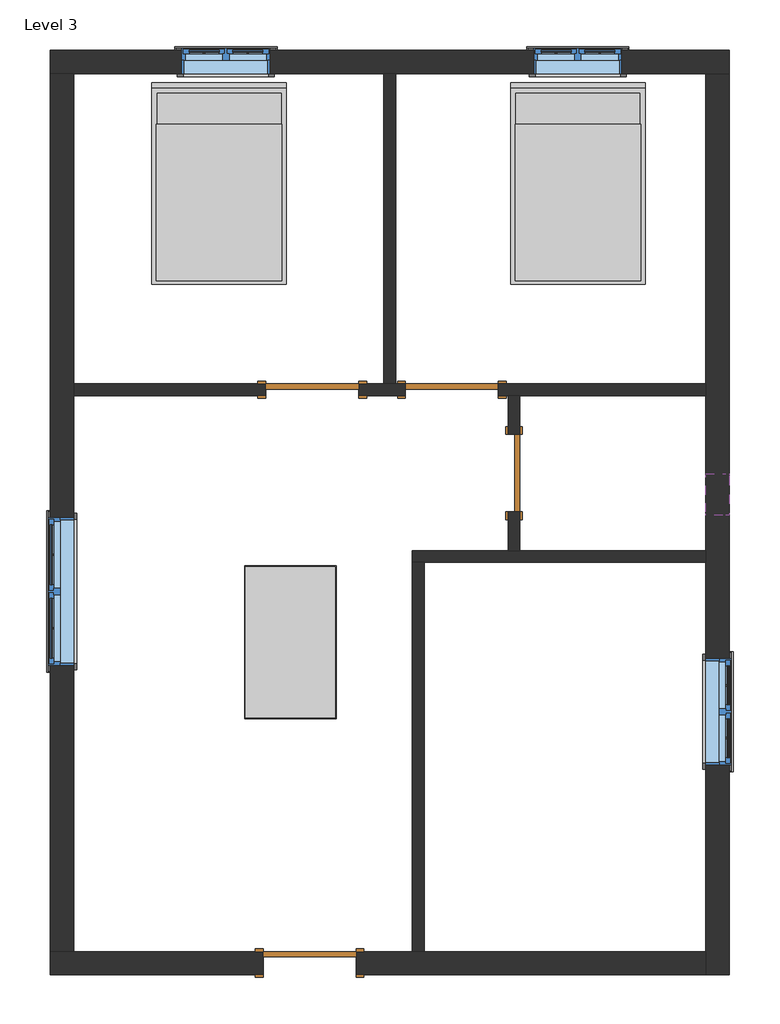
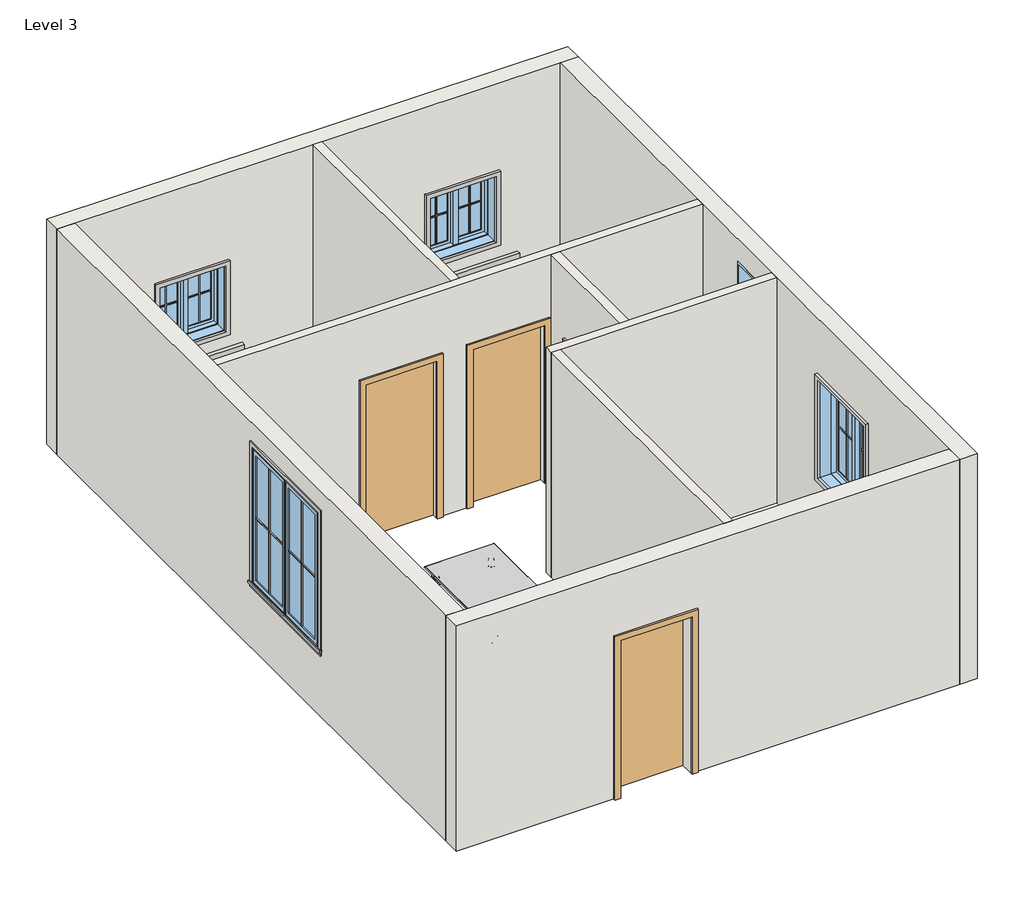
# One storey, incomplete: 16 proxies, 9 walls, 5 windows, 4 doors, 3 furniture elements.
"""IFC4 building model written with IfcOpenShell, lengths in millimetres."""

from ifc_helpers import new_model, si_unit, frame, origin, place, context, project, spatial, polyline, outline, extrude, faceted_brep, transform, mapped, element, save
from components import muntin_pattern_2x2_muntin_pattern_2x2_b3fe6957, muntin_pattern_2x2_muntin_pattern_2x2_3e0ecaf2, muntin_pattern_2x2_muntin_pattern_2x2_bff912c5, muntin_pattern_2x2_muntin_pattern_2x2_c2194282, muntin_pattern_2x2_muntin_pattern_2x2_88bf7f41, muntin_pattern_2x2_muntin_pattern_2x2_3dfd0a47, trim_window_exterior_flat_with_sill_41619996, trim_window_exterior_flat_with_sill_e04b3088, trim_window_exterior_flat_with_sill_4930676f, trim_window_interior_flat_picture_frame_51c85655, trim_window_interior_flat_picture_frame_2a7685fe, trim_window_interior_flat_picture_frame_dd064338, door_f2b275c1, door_e5f9f3c4, door_305aa2a5, door_0ca8825f, bed_17739_bed_17739_15c61121, dining_table_14755_dining_table_14755_d89cb775, window_aa618e30, window_339605e1, window_c95ebb39, window_9ac97e1a

model = new_model("IFC4")

# Units and contexts
model_context = context("Model", 3, world=origin())
ifc_project = project(units=[si_unit("LENGTHUNIT", "METRE", prefix="MILLI")], contexts=[model_context])

# Site, building, storey
site = spatial("IfcSite", under=ifc_project)
building = spatial("IfcBuilding", under=site)
storey = spatial("IfcBuildingStorey", under=building, Name="Level 3", Elevation=3200.4)

# Proxies
placement = place(None, origin())
muntin_pattern_2x2_muntin_pattern_2x2_shape = muntin_pattern_2x2_muntin_pattern_2x2_b3fe6957(model_context)
element("IfcBuildingElementProxy", 1, Name="Muntin Pattern_2x2 : Muntin Pattern_2x2", ObjectType="Muntin Pattern_2x2 : Muntin Pattern_2x2", at=placement, inside=storey, context=model_context, shape_type="MappedRepresentation", body=[
    mapped(muntin_pattern_2x2_muntin_pattern_2x2_shape, transform((-3079.2790084, 5068.9185985, 4184.65), x_axis=(1.0, 0.0, 0.0), y_axis=(0.0, 1.0, 0.0), z_axis=(0.0, 0.0, 1.0))),
])
element("IfcBuildingElementProxy", 2, Name="Muntin Pattern_2x2 : Muntin Pattern_2x2", ObjectType="Muntin Pattern_2x2 : Muntin Pattern_2x2", at=placement, inside=storey, context=model_context, shape_type="MappedRepresentation", body=[
    mapped(muntin_pattern_2x2_muntin_pattern_2x2_shape, transform((378.2959916, 5068.9185985, 4184.65), x_axis=(1.0, 0.0, 0.0), y_axis=(0.0, 1.0, 0.0), z_axis=(0.0, 0.0, 1.0))),
])
muntin_pattern_2x2_muntin_pattern_2x2_2_shape = muntin_pattern_2x2_muntin_pattern_2x2_3e0ecaf2(model_context)
element("IfcBuildingElementProxy", 3, Name="Muntin Pattern_2x2 : Muntin Pattern_2x2", ObjectType="Muntin Pattern_2x2 : Muntin Pattern_2x2", at=placement, inside=storey, context=model_context, shape_type="MappedRepresentation", body=[
    mapped(muntin_pattern_2x2_muntin_pattern_2x2_2_shape, transform((-2650.6540084, 5068.9185985, 4184.65), x_axis=(-1.0, 0.0, 0.0), y_axis=(0.0, -1.0, 0.0), z_axis=(0.0, 0.0, 1.0))),
])
element("IfcBuildingElementProxy", 4, Name="Muntin Pattern_2x2 : Muntin Pattern_2x2", ObjectType="Muntin Pattern_2x2 : Muntin Pattern_2x2", at=placement, inside=storey, context=model_context, shape_type="MappedRepresentation", body=[
    mapped(muntin_pattern_2x2_muntin_pattern_2x2_2_shape, transform((806.9209916, 5068.9185985, 4184.65), x_axis=(-1.0, 0.0, 0.0), y_axis=(0.0, -1.0, 0.0), z_axis=(0.0, 0.0, 1.0))),
])
muntin_pattern_2x2_muntin_pattern_2x2_3_shape = muntin_pattern_2x2_muntin_pattern_2x2_bff912c5(model_context)
element("IfcBuildingElementProxy", 5, Name="Muntin Pattern_2x2 : Muntin Pattern_2x2", ObjectType="Muntin Pattern_2x2 : Muntin Pattern_2x2", at=placement, inside=storey, context=model_context, shape_type="MappedRepresentation", body=[
    mapped(muntin_pattern_2x2_muntin_pattern_2x2_3_shape, transform((-4579.4665084, -596.8689015, 4184.65), x_axis=(0.0, 1.0, 0.0), y_axis=(-1.0, 0.0, 0.0), z_axis=(0.0, 0.0, 1.0))),
])
muntin_pattern_2x2_muntin_pattern_2x2_4_shape = muntin_pattern_2x2_muntin_pattern_2x2_c2194282(model_context)
element("IfcBuildingElementProxy", 6, Name="Muntin Pattern_2x2 : Muntin Pattern_2x2", ObjectType="Muntin Pattern_2x2 : Muntin Pattern_2x2", at=placement, inside=storey, context=model_context, shape_type="MappedRepresentation", body=[
    mapped(muntin_pattern_2x2_muntin_pattern_2x2_4_shape, transform((-4579.4665084, 123.8560985, 4184.65), x_axis=(0.0, -1.0, 0.0), y_axis=(1.0, 0.0, 0.0), z_axis=(0.0, 0.0, 1.0))),
])
muntin_pattern_2x2_muntin_pattern_2x2_5_shape = muntin_pattern_2x2_muntin_pattern_2x2_88bf7f41(model_context)
element("IfcBuildingElementProxy", 7, Name="Muntin Pattern_2x2 : Muntin Pattern_2x2", ObjectType="Muntin Pattern_2x2 : Muntin Pattern_2x2", at=placement, inside=storey, context=model_context, shape_type="MappedRepresentation", body=[
    mapped(muntin_pattern_2x2_muntin_pattern_2x2_5_shape, transform((2068.9834916, -1158.8439015, 4184.65), x_axis=(0.0, -1.0, 0.0), y_axis=(1.0, 0.0, 0.0), z_axis=(0.0, 0.0, 1.0))),
])
muntin_pattern_2x2_muntin_pattern_2x2_6_shape = muntin_pattern_2x2_muntin_pattern_2x2_3dfd0a47(model_context)
element("IfcBuildingElementProxy", 8, Name="Muntin Pattern_2x2 : Muntin Pattern_2x2", ObjectType="Muntin Pattern_2x2 : Muntin Pattern_2x2", at=placement, inside=storey, context=model_context, shape_type="MappedRepresentation", body=[
    mapped(muntin_pattern_2x2_muntin_pattern_2x2_6_shape, transform((2068.9834916, -1676.3689015, 4184.65), x_axis=(0.0, 1.0, 0.0), y_axis=(-1.0, 0.0, 0.0), z_axis=(0.0, 0.0, 1.0))),
])
trim_window_exterior_flat_with_sill_shape = trim_window_exterior_flat_with_sill_41619996(model_context)
element("IfcBuildingElementProxy", 9, Name="Trim-Window-Exterior-Flat : with Sill", ObjectType="Trim-Window-Exterior-Flat : with Sill", at=placement, inside=storey, context=model_context, shape_type="MappedRepresentation", body=[
    mapped(trim_window_exterior_flat_with_sill_shape, transform((-2864.9665084, 5078.4435985, 5029.2), x_axis=(-1.0, 0.0, 0.0), y_axis=(0.0, 0.0, 1.0), z_axis=(0.0, 1.0, 0.0))),
])
element("IfcBuildingElementProxy", 10, Name="Trim-Window-Exterior-Flat : with Sill", ObjectType="Trim-Window-Exterior-Flat : with Sill", at=placement, inside=storey, context=model_context, shape_type="MappedRepresentation", body=[
    mapped(trim_window_exterior_flat_with_sill_shape, transform((592.6084916, 5078.4435985, 5029.2), x_axis=(-1.0, 0.0, 0.0), y_axis=(0.0, 0.0, 1.0), z_axis=(0.0, 1.0, 0.0))),
])
trim_window_exterior_flat_with_sill_2_shape = trim_window_exterior_flat_with_sill_e04b3088(model_context)
element("IfcBuildingElementProxy", 11, Name="Trim-Window-Exterior-Flat : with Sill", ObjectType="Trim-Window-Exterior-Flat : with Sill", at=placement, inside=storey, context=model_context, shape_type="MappedRepresentation", body=[
    mapped(trim_window_exterior_flat_with_sill_2_shape, transform((-4588.9915084, -236.5064015, 5943.6), x_axis=(0.0, -1.0, 0.0), y_axis=(0.0, 0.0, 1.0), z_axis=(-1.0, 0.0, 0.0))),
])
trim_window_exterior_flat_with_sill_3_shape = trim_window_exterior_flat_with_sill_4930676f(model_context)
element("IfcBuildingElementProxy", 12, Name="Trim-Window-Exterior-Flat : with Sill", ObjectType="Trim-Window-Exterior-Flat : with Sill", at=placement, inside=storey, context=model_context, shape_type="MappedRepresentation", body=[
    mapped(trim_window_exterior_flat_with_sill_3_shape, transform((2078.5084916, -1417.6064015, 5461.0), x_axis=(0.0, 1.0, 0.0), y_axis=(0.0, 0.0, 1.0), z_axis=(1.0, 0.0, 0.0))),
])
trim_window_interior_flat_picture_frame_shape = trim_window_interior_flat_picture_frame_51c85655(model_context)
element("IfcBuildingElementProxy", 13, Name="Trim-Window-Interior-Flat : Picture Frame", ObjectType="Trim-Window-Interior-Flat : Picture Frame", at=placement, inside=storey, context=model_context, shape_type="MappedRepresentation", body=[
    mapped(trim_window_interior_flat_picture_frame_shape, transform((-2864.9665084, 4849.8435985, 5029.2), x_axis=(1.0, 0.0, 0.0), y_axis=(0.0, 0.0, 1.0), z_axis=(0.0, -1.0, 0.0))),
])
element("IfcBuildingElementProxy", 14, Name="Trim-Window-Interior-Flat : Picture Frame", ObjectType="Trim-Window-Interior-Flat : Picture Frame", at=placement, inside=storey, context=model_context, shape_type="MappedRepresentation", body=[
    mapped(trim_window_interior_flat_picture_frame_shape, transform((592.6084916, 4849.8435985, 5029.2), x_axis=(1.0, 0.0, 0.0), y_axis=(0.0, 0.0, 1.0), z_axis=(0.0, -1.0, 0.0))),
])
trim_window_interior_flat_picture_frame_2_shape = trim_window_interior_flat_picture_frame_2a7685fe(model_context)
element("IfcBuildingElementProxy", 15, Name="Trim-Window-Interior-Flat : Picture Frame", ObjectType="Trim-Window-Interior-Flat : Picture Frame", at=placement, inside=storey, context=model_context, shape_type="MappedRepresentation", body=[
    mapped(trim_window_interior_flat_picture_frame_2_shape, transform((-4360.3915084, -236.5064015, 5943.6), x_axis=(0.0, 1.0, 0.0), y_axis=(0.0, 0.0, 1.0), z_axis=(1.0, 0.0, 0.0))),
])
trim_window_interior_flat_picture_frame_3_shape = trim_window_interior_flat_picture_frame_dd064338(model_context)
element("IfcBuildingElementProxy", 16, Name="Trim-Window-Interior-Flat : Picture Frame", ObjectType="Trim-Window-Interior-Flat : Picture Frame", at=placement, inside=storey, context=model_context, shape_type="MappedRepresentation", body=[
    mapped(trim_window_interior_flat_picture_frame_3_shape, transform((1849.9084916, -1417.6064015, 5461.0), x_axis=(0.0, -1.0, 0.0), y_axis=(0.0, 0.0, 1.0), z_axis=(-1.0, 0.0, 0.0))),
])

# Doors
door_shape = door_f2b275c1(model_context)
element("IfcDoor", 17, ObjectType="Single-Flush : 30\" x 80\"", at=placement, inside=storey, context=model_context, shape_type="MappedRepresentation", body=[
    mapped(door_shape, transform((-36.0415084, 925.5435985, 3200.4), x_axis=(0.0, 1.0, 0.0), y_axis=(-1.0, 0.0, 0.0), z_axis=(0.0, 0.0, 1.0))),
])
door_2_shape = door_e5f9f3c4(model_context)
element("IfcDoor", 18, ObjectType="Single-Flush : 36\" x 84\"", at=placement, inside=storey, context=model_context, shape_type="MappedRepresentation", body=[
    mapped(door_2_shape, transform((-2017.2415084, 1744.6935985, 3200.4), x_axis=(1.0, 0.0, 0.0), y_axis=(0.0, 1.0, 0.0), z_axis=(0.0, 0.0, 1.0))),
])
door_3_shape = door_305aa2a5(model_context)
element("IfcDoor", 19, ObjectType="Single-Flush : 36\" x 84\"", at=placement, inside=storey, context=model_context, shape_type="MappedRepresentation", body=[
    mapped(door_3_shape, transform((-645.6415084, 1744.6935985, 3200.4), x_axis=(-1.0, 0.0, 0.0), y_axis=(0.0, -1.0, 0.0), z_axis=(0.0, 0.0, 1.0))),
])
door_4_shape = door_0ca8825f(model_context)
element("IfcDoor", 20, ObjectType="Single-Flush : 36\" x 84\"", at=placement, inside=storey, context=model_context, shape_type="MappedRepresentation", body=[
    mapped(door_4_shape, transform((-2042.6415084, -3887.7564015, 3200.4), x_axis=(1.0, 0.0, 0.0), y_axis=(0.0, 1.0, 0.0), z_axis=(0.0, 0.0, 1.0))),
])

# Furniture
bed_17739_bed_17739_shape = bed_17739_bed_17739_15c61121(model_context)
element("IfcFurniture", 21, ObjectType="Bed_17739 : Bed_17739", at=placement, inside=storey, context=model_context, shape_type="MappedRepresentation", body=[
    mapped(bed_17739_bed_17739_shape, transform((-2931.6415084, 3744.9435985, 3200.4), x_axis=(1.0, 0.0, 0.0), y_axis=(0.0, 1.0, 0.0), z_axis=(0.0, 0.0, 1.0))),
])
element("IfcFurniture", 22, ObjectType="Bed_17739 : Bed_17739", at=placement, inside=storey, context=model_context, shape_type="MappedRepresentation", body=[
    mapped(bed_17739_bed_17739_shape, transform((592.6084916, 3744.9435985, 3200.4), x_axis=(1.0, 0.0, 0.0), y_axis=(0.0, 1.0, 0.0), z_axis=(0.0, 0.0, 1.0))),
])
dining_table_14755_dining_table_14755_shape = dining_table_14755_dining_table_14755_d89cb775(model_context)
element("IfcFurniture", 23, ObjectType="Dining_table_14755 : Dining_table_14755", at=placement, inside=storey, context=model_context, shape_type="MappedRepresentation", body=[
    mapped(dining_table_14755_dining_table_14755_shape, transform((-1781.6222109, -1485.4350296, 3200.4), x_axis=(0.0, 1.0, 0.0), y_axis=(-1.0, 0.0, 0.0), z_axis=(0.0, 0.0, 1.0))),
])

# Walls
element("IfcWall", 24, ObjectType="WALL4.5\"", at=placement, inside=storey, context=model_context, shape_type="Brep", body=[
    faceted_brep([(-1560.0415084, 1687.5435985, 3200.4), (-1102.8415084, 1687.5435985, 3200.4), (-1102.8415084, 1687.5435985, 5334.0), (-188.4415084, 1687.5435985, 5334.0), (-188.4415084, 1687.5435985, 3200.4), (-93.1915084, 1687.5435985, 3200.4), (21.1084916, 1687.5435985, 3200.4), (1849.9084916, 1687.5435985, 3200.4), (1849.9084916, 1687.5435985, 6248.4), (21.1084916, 1687.5435985, 6248.4), (-93.1915084, 1687.5435985, 6248.4), (-4360.3915084, 1687.5435985, 6248.4), (-4360.3915084, 1687.5435985, 3200.4), (-2474.4415084, 1687.5435985, 3200.4), (-2474.4415084, 1687.5435985, 5334.0), (-1560.0415084, 1687.5435985, 5334.0), (-1102.8415084, 1801.8435985, 5334.0), (-1102.8415084, 1801.8435985, 3200.4), (-1198.0915084, 1801.8435985, 3200.4), (-1312.3915084, 1801.8435985, 3200.4), (-1560.0415084, 1801.8435985, 3200.4), (-1560.0415084, 1801.8435985, 5334.0), (-2474.4415084, 1801.8435985, 5334.0), (-2474.4415084, 1801.8435985, 3200.4), (-4360.3915084, 1801.8435985, 3200.4), (-4360.3915084, 1801.8435985, 6248.4), (-1312.3915084, 1801.8435985, 6248.4), (-1198.0915084, 1801.8435985, 6248.4), (1849.9084916, 1801.8435985, 6248.4), (1849.9084916, 1801.8435985, 3200.4), (-188.4415084, 1801.8435985, 3200.4), (-188.4415084, 1801.8435985, 5334.0)], [[[0, 1, 2, 3, 4, 5, 6, 7, 8, 9, 10, 11, 12, 13, 14, 15]], [[16, 17, 18, 19, 20, 21, 22, 23, 24, 25, 26, 27, 28, 29, 30, 31]], [[13, 12, 24, 23]], [[30, 29, 7, 6, 5, 4]], [[20, 19, 18, 17, 1, 0]], [[8, 7, 29, 28]], [[12, 11, 25, 24]], [[21, 20, 0, 15]], [[22, 21, 15, 14]], [[23, 22, 14, 13]], [[2, 1, 17, 16]], [[3, 2, 16, 31]], [[4, 3, 31, 30]], [[11, 10, 9, 8, 28, 27, 26, 25]]]),
])
element("IfcWall", 25, ObjectType="WALL4.5\"", at=placement, inside=storey, context=model_context, shape_type="SweptSolid", body=[
    extrude(outline(polyline([(-1312.3915084, 1801.8435985), (-1312.3915084, 4849.8435985), (-1198.0915084, 4849.8435985), (-1198.0915084, 1801.8435985), (-1312.3915084, 1801.8435985)])), frame((0.0, 0.0, 3200.4), z_axis=(0.0, 0.0, 1.0), x_axis=(1.0, 0.0, 0.0)), (0.0, 0.0, 1.0), 3048.0),
])
element("IfcWall", 26, ObjectType="WALL4.5\"", at=placement, inside=storey, context=model_context, shape_type="SweptSolid", body=[
    extrude(outline(polyline([(1687.5435985, 3200.4), (1306.5435985, 3200.4), (1306.5435985, 5232.4), (544.5435985, 5232.4), (544.5435985, 3200.4), (163.5435985, 3200.4), (163.5435985, 6248.4), (1687.5435985, 6248.4), (1687.5435985, 3200.4)])), frame((-93.1915084, 0.0, 0.0), z_axis=(1.0, 0.0, 0.0), x_axis=(0.0, 1.0, 0.0)), (0.0, 0.0, 1.0), 114.3),
])
element("IfcWall", 27, ObjectType="WALL4.5\"", at=placement, inside=storey, context=model_context, shape_type="Brep", body=[
    faceted_brep([(1849.9084916, 163.5435985, 3200.4), (21.1084916, 163.5435985, 3200.4), (-93.1915084, 163.5435985, 3200.4), (-1032.9915084, 163.5435985, 3200.4), (-1032.9915084, 163.5435985, 6248.4), (-93.1915084, 163.5435985, 6248.4), (21.1084916, 163.5435985, 6248.4), (1849.9084916, 163.5435985, 6248.4), (1849.9084916, 49.2435985, 3200.4), (1849.9084916, 49.2435985, 6248.4), (-918.6915084, 49.2435985, 6248.4), (-1032.9915084, 49.2435985, 6248.4), (-1032.9915084, 49.2435985, 3200.4), (-918.6915084, 49.2435985, 3200.4)], [[[0, 1, 2, 3, 4, 5, 6, 7]], [[8, 9, 10, 11, 12, 13]], [[3, 2, 1, 0, 8, 13, 12]], [[0, 7, 9, 8]], [[4, 3, 12, 11]], [[7, 6, 5, 4, 11, 10, 9]]]),
])
element("IfcWall", 28, ObjectType="WALL4.5\"", at=placement, inside=storey, context=model_context, shape_type="SweptSolid", body=[
    extrude(outline(polyline([(-1032.9915084, -3773.4564015), (-1032.9915084, 49.2435985), (-918.6915084, 49.2435985), (-918.6915084, -3773.4564015), (-1032.9915084, -3773.4564015)])), frame((0.0, 0.0, 3200.4), z_axis=(0.0, 0.0, 1.0), x_axis=(1.0, 0.0, 0.0)), (0.0, 0.0, 1.0), 3048.0),
])
element("IfcWall", 29, ObjectType="WALL9\"", at=placement, inside=storey, context=model_context, shape_type="Brep", body=[
    faceted_brep([(-4588.9915084, 4849.8435985, 3200.4), (-4360.3915084, 4849.8435985, 3200.4), (-1312.3915084, 4849.8435985, 3200.4), (-1198.0915084, 4849.8435985, 3200.4), (1849.9084916, 4849.8435985, 3200.4), (2078.5084916, 4849.8435985, 3200.4), (2078.5084916, 4849.8435985, 6248.4), (1849.9084916, 4849.8435985, 6248.4), (-1198.0915084, 4849.8435985, 6248.4), (-1312.3915084, 4849.8435985, 6248.4), (-4360.3915084, 4849.8435985, 6248.4), (-4588.9915084, 4849.8435985, 6248.4), (-2433.1665084, 4849.8435985, 5029.2), (-2433.1665084, 4849.8435985, 4114.8), (-3296.7665084, 4849.8435985, 4114.8), (-3296.7665084, 4849.8435985, 5029.2), (1024.4084916, 4849.8435985, 5029.2), (1024.4084916, 4849.8435985, 4114.8), (160.8084916, 4849.8435985, 4114.8), (160.8084916, 4849.8435985, 5029.2), (-4588.9915084, 5078.4435985, 3200.4), (-4588.9915084, 5078.4435985, 6248.4), (2078.5084916, 5078.4435985, 6248.4), (2078.5084916, 5078.4435985, 3200.4), (-2433.1665084, 5078.4435985, 5029.2), (-3296.7665084, 5078.4435985, 5029.2), (-3296.7665084, 5078.4435985, 4114.8), (-2433.1665084, 5078.4435985, 4114.8), (1024.4084916, 5078.4435985, 5029.2), (160.8084916, 5078.4435985, 5029.2), (160.8084916, 5078.4435985, 4114.8), (1024.4084916, 5078.4435985, 4114.8)], [[[0, 1, 2, 3, 4, 5, 6, 7, 8, 9, 10, 11], [12, 13, 14, 15], [16, 17, 18, 19]], [[20, 21, 22, 23], [24, 25, 26, 27], [28, 29, 30, 31]], [[5, 4, 3, 2, 1, 0, 20, 23]], [[6, 5, 23, 22]], [[0, 11, 21, 20]], [[13, 12, 24, 27]], [[14, 13, 27, 26]], [[15, 14, 26, 25]], [[12, 15, 25, 24]], [[17, 16, 28, 31]], [[18, 17, 31, 30]], [[19, 18, 30, 29]], [[16, 19, 29, 28]], [[11, 10, 9, 8, 7, 6, 22, 21]]]),
])
element("IfcWall", 30, ObjectType="WALL9\"", at=placement, inside=storey, context=model_context, shape_type="Brep", body=[
    faceted_brep([(1849.9084916, 4849.8435985, 3200.4), (1849.9084916, 1801.8435985, 3200.4), (1849.9084916, 1687.5435985, 3200.4), (1849.9084916, 163.5435985, 3200.4), (1849.9084916, 49.2435985, 3200.4), (1849.9084916, -3773.4564015, 3200.4), (1849.9084916, -4002.0564015, 3200.4), (1849.9084916, -4002.0564015, 6248.4), (1849.9084916, -3773.4564015, 6248.4), (1849.9084916, 49.2435985, 6248.4), (1849.9084916, 163.5435985, 6248.4), (1849.9084916, 1687.5435985, 6248.4), (1849.9084916, 1801.8435985, 6248.4), (1849.9084916, 4849.8435985, 6248.4), (1849.9084916, -1938.3064015, 5461.0), (1849.9084916, -1938.3064015, 4114.8), (1849.9084916, -896.9064015, 4114.8), (1849.9084916, -896.9064015, 5461.0), (1849.9084916, 512.7935985, 5943.6), (1849.9084916, 512.7935985, 5334.0), (1849.9084916, 919.1935985, 5334.0), (1849.9084916, 919.1935985, 5943.6), (2078.5084916, 4849.8435985, 3200.4), (2078.5084916, 4849.8435985, 6248.4), (2078.5084916, -4002.0564015, 6248.4), (2078.5084916, -4002.0564015, 3200.4), (2078.5084916, -1938.3064015, 5461.0), (2078.5084916, -896.9064015, 5461.0), (2078.5084916, -896.9064015, 4114.8), (2078.5084916, -1938.3064015, 4114.8), (2078.5084916, 512.7935985, 5943.6), (2078.5084916, 919.1935985, 5943.6), (2078.5084916, 919.1935985, 5334.0), (2078.5084916, 512.7935985, 5334.0)], [[[0, 1, 2, 3, 4, 5, 6, 7, 8, 9, 10, 11, 12, 13], [14, 15, 16, 17], [18, 19, 20, 21]], [[22, 23, 24, 25], [26, 27, 28, 29], [30, 31, 32, 33]], [[6, 5, 4, 3, 2, 1, 0, 22, 25]], [[0, 13, 23, 22]], [[7, 6, 25, 24]], [[15, 14, 26, 29]], [[16, 15, 29, 28]], [[17, 16, 28, 27]], [[14, 17, 27, 26]], [[19, 18, 30, 33]], [[20, 19, 33, 32]], [[21, 20, 32, 31]], [[18, 21, 31, 30]], [[13, 12, 11, 10, 9, 8, 7, 24, 23]]]),
])
element("IfcWall", 31, ObjectType="WALL9\"", at=placement, inside=storey, context=model_context, shape_type="Brep", body=[
    faceted_brep([(1849.9084916, -3773.4564015, 3200.4), (-918.6915084, -3773.4564015, 3200.4), (-1032.9915084, -3773.4564015, 3200.4), (-1585.4415084, -3773.4564015, 3200.4), (-1585.4415084, -3773.4564015, 5334.0), (-2499.8415084, -3773.4564015, 5334.0), (-2499.8415084, -3773.4564015, 3200.4), (-4360.3915084, -3773.4564015, 3200.4), (-4588.9915084, -3773.4564015, 3200.4), (-4588.9915084, -3773.4564015, 6248.4), (-4360.3915084, -3773.4564015, 6248.4), (-1032.9915084, -3773.4564015, 6248.4), (-918.6915084, -3773.4564015, 6248.4), (1849.9084916, -3773.4564015, 6248.4), (-1585.4415084, -4002.0564015, 5334.0), (-1585.4415084, -4002.0564015, 3200.4), (1849.9084916, -4002.0564015, 3200.4), (1849.9084916, -4002.0564015, 6248.4), (-4588.9915084, -4002.0564015, 6248.4), (-4588.9915084, -4002.0564015, 3200.4), (-2499.8415084, -4002.0564015, 3200.4), (-2499.8415084, -4002.0564015, 5334.0)], [[[0, 1, 2, 3, 4, 5, 6, 7, 8, 9, 10, 11, 12, 13]], [[14, 15, 16, 17, 18, 19, 20, 21]], [[20, 19, 8, 7, 6]], [[16, 15, 3, 2, 1, 0]], [[0, 13, 17, 16]], [[9, 8, 19, 18]], [[4, 3, 15, 14]], [[5, 4, 14, 21]], [[6, 5, 21, 20]], [[13, 12, 11, 10, 9, 18, 17]]]),
])
element("IfcWall", 32, ObjectType="WALL9\"", at=placement, inside=storey, context=model_context, shape_type="Brep", body=[
    faceted_brep([(-4360.3915084, -3773.4564015, 3200.4), (-4360.3915084, 1687.5435985, 3200.4), (-4360.3915084, 1801.8435985, 3200.4), (-4360.3915084, 4849.8435985, 3200.4), (-4360.3915084, 4849.8435985, 6248.4), (-4360.3915084, 1801.8435985, 6248.4), (-4360.3915084, 1687.5435985, 6248.4), (-4360.3915084, -3773.4564015, 6248.4), (-4360.3915084, 487.3935985, 5943.6), (-4360.3915084, 487.3935985, 4114.8), (-4360.3915084, -960.4064015, 4114.8), (-4360.3915084, -960.4064015, 5943.6), (-4588.9915084, -3773.4564015, 3200.4), (-4588.9915084, -3773.4564015, 6248.4), (-4588.9915084, 4849.8435985, 6248.4), (-4588.9915084, 4849.8435985, 3200.4), (-4588.9915084, 487.3935985, 5943.6), (-4588.9915084, -960.4064015, 5943.6), (-4588.9915084, -960.4064015, 4114.8), (-4588.9915084, 487.3935985, 4114.8)], [[[0, 1, 2, 3, 4, 5, 6, 7], [8, 9, 10, 11]], [[12, 13, 14, 15], [16, 17, 18, 19]], [[3, 2, 1, 0, 12, 15]], [[0, 7, 13, 12]], [[4, 3, 15, 14]], [[9, 8, 16, 19]], [[10, 9, 19, 18]], [[11, 10, 18, 17]], [[8, 11, 17, 16]], [[7, 6, 5, 4, 14, 13]]]),
])

# Windows
window_shape = window_aa618e30(model_context)
element("IfcWindow", 33, ObjectType="Fixed : 16\" x 24\"", at=placement, inside=storey, context=model_context, shape_type="MappedRepresentation", body=[
    mapped(window_shape, transform((1964.2084916, 677.8935985, 4419.6), x_axis=(0.0, -1.0, 0.0), y_axis=(1.0, 0.0, 0.0), z_axis=(0.0, 0.0, 1.0))),
])
window_2_shape = window_339605e1(model_context)
element("IfcWindow", 34, ObjectType="Window-Casement-Double : 34\" x 36\"", at=placement, inside=storey, context=model_context, shape_type="MappedRepresentation", body=[
    mapped(window_2_shape, transform((-2864.9665084, 4964.1435985, 3200.4), x_axis=(1.0, 0.0, 0.0), y_axis=(0.0, 1.0, 0.0), z_axis=(0.0, 0.0, 1.0))),
])
element("IfcWindow", 35, ObjectType="Window-Casement-Double : 34\" x 36\"", at=placement, inside=storey, context=model_context, shape_type="MappedRepresentation", body=[
    mapped(window_2_shape, transform((592.6084916, 4964.1435985, 3200.4), x_axis=(1.0, 0.0, 0.0), y_axis=(0.0, 1.0, 0.0), z_axis=(0.0, 0.0, 1.0))),
])
window_3_shape = window_c95ebb39(model_context)
element("IfcWindow", 36, ObjectType="Window-Casement-Double : 41\" x 53\"", at=placement, inside=storey, context=model_context, shape_type="MappedRepresentation", body=[
    mapped(window_3_shape, transform((1964.2084916, -1417.6064015, 3200.4), x_axis=(0.0, -1.0, 0.0), y_axis=(1.0, 0.0, 0.0), z_axis=(0.0, 0.0, 1.0))),
])
window_4_shape = window_9ac97e1a(model_context)
element("IfcWindow", 37, ObjectType="Window-Casement-Double : 57\" x 72\"", at=placement, inside=storey, context=model_context, shape_type="MappedRepresentation", body=[
    mapped(window_4_shape, transform((-4474.6915084, -236.5064015, 3200.4), x_axis=(0.0, 1.0, 0.0), y_axis=(-1.0, 0.0, 0.0), z_axis=(0.0, 0.0, 1.0))),
])

save(model, "model.ifc")

# Revit data of these elements
# Type "Muntin Pattern_2x2 : Muntin Pattern_2x2"
#   Width [instance default] = 4' - 0"
#   Thickness = 0' - 0 1/2"
#   Height [instance default] = 4' - 0"
#   Distance = 0' - 0 3/4"
#   Interior Material [instance default] = none
#   Exterior Material [instance default] = none
#   Default Elevation = 0
# Type "Trim-Window-Exterior-Flat : with Sill"
#   Trim Width = 0' - 2 1/4"
#   Trim Thickness_Picture Frame = 0' - 1 1/4"
#   Trim Thickness_with Sill = 0' - 0 3/4"
#   Sill Thickness = 0' - 1 1/4"
#   Opening Width [instance default] = 2' - 0"
#   Opening Height [instance default] = 3' - 0"
#   Default Elevation = 4' - 0"
#   Sill = yes
#   Picture Frame = no
#   Trim Material [instance default] = none
# Type "Trim-Window-Interior-Flat : Picture Frame"
#   Trim Thickness_Picture Frame = 0' - 1 1/4"
#   Trim Width = 0' - 2 1/4"
#   Trim Thickness_with Sill = 0' - 0 3/4"
#   Sill Thickness = 0' - 1 1/4"
#   Opening Width [instance default] = 2' - 0"
#   Opening Height [instance default] = 3' - 0"
#   Default Elevation = 4' - 0"
#   Sill = no
#   Picture Frame = yes
#   Trim Material [instance default] = none
# Type "Single-Flush : 30\" x 80\""
#   Type Mark = "5"
#   Construction Type Id = "MDOOR"
#   Assembly Code = "C1020"
#   Analytic Construction = "Metal"
#   Thickness = 0' - 2"
#   Heat Transfer Coefficient (U) = 0.651978 BTU/(h·ft²·°F)
#   Height = 6' - 8"
#   Trim Projection Ext = 0' - 1"
#   Trim Projection Int = 0' - 1"
#   Trim Width = 0' - 3"
#   Width = 2' - 6"
#   Define Thermal Properties by = 1
#   Define Thermal Properties by = 1
#   Door Material = Door - Panel
#   Frame Material = Door - Frame
#   Visual Light Transmittance = 0
#   Solar Heat Gain Coefficient = 0
#   Function = (empty or 0)
#   Wall Closure = (empty or 0)
# Type "Single-Flush : 36\" x 84\""
#   Type Mark = "1"
#   Construction Type Id = "MDOOR"
#   Assembly Code = "C1020"
#   Analytic Construction = "Metal"
#   Thickness = 0' - 2"
#   Heat Transfer Coefficient (U) = 0.651978 BTU/(h·ft²·°F)
#   Height = 7' - 0"
#   Trim Projection Ext = 0' - 1"
#   Trim Projection Int = 0' - 1"
#   Trim Width = 0' - 3"
#   Width = 3' - 0"
#   Define Thermal Properties by = 1
#   Define Thermal Properties by = 1
#   Door Material = Door - Panel
#   Frame Material = Door - Frame
#   Visual Light Transmittance = 0
#   Solar Heat Gain Coefficient = 0
#   Function = (empty or 0)
#   Wall Closure = (empty or 0)
# Type "Bed_17739 : Bed_17739"
#   Default Elevation = 0
# Type "Dining_table_14755 : Dining_table_14755"
#   Lengte [instance default] = 4' - 11.05512"
#   Breedte [instance default] = 2' - 11.43307"
#   Tafelblad = none
#   Poten = none
#   Default Elevation = 0
# Type "WALL4.5\""
#   Assembly Code = "B2010"
#   Layers, outside or top first: 0' - 4 1/2" no material (function 1)
# Type "WALL9\""
#   Assembly Code = "B2010"
#   Layers, outside or top first: 0' - 9" no material (function 1)
# Type "Fixed : 16\" x 24\""
#   Type Mark = "4"
#   Construction Type Id = "GSP4R"
#   Assembly Code = "B2020100"
#   Analytic Construction = "1/8 in Pilkington single glazing"
#   Visual Light Transmittance = 0.9
#   Solar Heat Gain Coefficient = 0.78
#   Heat Transfer Coefficient (U) = 0.6496 BTU/(h·ft²·°F)
#   Height = 2' - 0"
#   Default Sill Height = 3' - 0"
#   Width = 1' - 4"
#   Window Inset = 0' - 0 3/4"
#   Define Thermal Properties by = 1
#   Define Thermal Properties by = 1
#   Glass Pane Material = Glass
#   Sash Material = Sash
#   Wall Closure = (empty or 0)
# Type "Window-Casement-Double : 34\" x 36\""
#   Type Mark = "14"
#   Fire Rating = "0.5h"
#   Assembly Code = "B2020100"
#   Analytic Construction = "Double glazing - domestic"
#   Frame Extension [instance default] = 0' - 0 1/4"
#   Window Inset [instance default] = 0' - 0"
#   Wall Thickness [instance default] = 0' - 6"
#   Interior Wall Closure [instance default] = 0' - 2 1/4"
#   Half Width = 1' - 5"
#   Visual Light Transmittance = 0.81
#   Thermal Resistance (R) = 1.8146 (h·ft²·°F)/BTU
#   Solar Heat Gain Coefficient = 0.76
#   Rough Width = 2' - 10 1/2"
#   Rough Height = 3' - 0 1/2"
#   Height = 3' - 0"
#   Heat Transfer Coefficient (U) = 0.5511 BTU/(h·ft²·°F)
#   Exterior Wall Closure [instance default] = 0' - 1 1/4"
#   Extension Jamb [instance default] = 0' - 2 1/4"
#   Default Sill Height = 3' - 0"
#   Width = 2' - 10"
#   Define Thermal Properties by = 0
#   Muntin Visibility = yes
#   Interior Trim Visibility [instance default] = yes
#   Exterior Trim Visibility [instance default] = yes
#   Extension Jamb Visibility [instance default] = yes
#   Interior Trim Material = Wood - Stained
#   Muntin Pattern = Muntin Pattern_2x2 : Muntin Pattern_2x2
#   Interior Trim = Trim-Window-Interior-Flat : Picture Frame
#   Interior Frame Material = Wood - Stained
#   Glass Panel Material = Glass
#   Exterior Trim Material = Clad - White
#   Exterior Trim = Trim-Window-Exterior-Flat : with Sill
#   Exterior Frame Material = Clad - White
#   Wall Closure = (empty or 0)
# Type "Window-Casement-Double : 41\" x 53\""
#   Type Mark = "15"
#   Fire Rating = "0.5h"
#   Assembly Code = "B2020100"
#   Analytic Construction = "Double glazing - domestic"
#   Frame Extension [instance default] = 0' - 0 1/4"
#   Window Inset [instance default] = 0' - 0"
#   Wall Thickness [instance default] = 0' - 6"
#   Interior Wall Closure [instance default] = 0' - 2 1/4"
#   Half Width = 1' - 8 1/2"
#   Visual Light Transmittance = 0.81
#   Thermal Resistance (R) = 1.8146 (h·ft²·°F)/BTU
#   Solar Heat Gain Coefficient = 0.76
#   Rough Width = 3' - 5 1/2"
#   Rough Height = 4' - 5 1/2"
#   Height = 4' - 5"
#   Heat Transfer Coefficient (U) = 0.5511 BTU/(h·ft²·°F)
#   Exterior Wall Closure [instance default] = 0' - 1 1/4"
#   Extension Jamb [instance default] = 0' - 2 1/4"
#   Default Sill Height = 3' - 0"
#   Width = 3' - 5"
#   Define Thermal Properties by = 0
#   Muntin Visibility = yes
#   Interior Trim Visibility [instance default] = yes
#   Exterior Trim Visibility [instance default] = yes
#   Extension Jamb Visibility [instance default] = yes
#   Interior Trim Material = Wood - Stained
#   Muntin Pattern = Muntin Pattern_2x2 : Muntin Pattern_2x2
#   Interior Trim = Trim-Window-Interior-Flat : Picture Frame
#   Interior Frame Material = Wood - Stained
#   Glass Panel Material = Glass
#   Exterior Trim Material = Clad - White
#   Exterior Trim = Trim-Window-Exterior-Flat : with Sill
#   Exterior Frame Material = Clad - White
#   Wall Closure = (empty or 0)
# Type "Window-Casement-Double : 57\" x 72\""
#   Type Mark = "17"
#   Fire Rating = "0.5h"
#   Assembly Code = "B2020100"
#   Analytic Construction = "Double glazing - domestic"
#   Frame Extension [instance default] = 0' - 0 1/4"
#   Window Inset [instance default] = 0' - 0"
#   Wall Thickness [instance default] = 0' - 6"
#   Interior Wall Closure [instance default] = 0' - 2 1/4"
#   Half Width = 2' - 4 1/2"
#   Visual Light Transmittance = 0.81
#   Thermal Resistance (R) = 1.8146 (h·ft²·°F)/BTU
#   Solar Heat Gain Coefficient = 0.76
#   Rough Width = 4' - 9 1/2"
#   Rough Height = 6' - 0 1/2"
#   Height = 6' - 0"
#   Heat Transfer Coefficient (U) = 0.5511 BTU/(h·ft²·°F)
#   Exterior Wall Closure [instance default] = 0' - 1 1/4"
#   Extension Jamb [instance default] = 0' - 2 1/4"
#   Default Sill Height = 3' - 0"
#   Width = 4' - 9"
#   Define Thermal Properties by = 0
#   Muntin Visibility = yes
#   Interior Trim Visibility [instance default] = yes
#   Exterior Trim Visibility [instance default] = yes
#   Extension Jamb Visibility [instance default] = yes
#   Interior Trim Material = Wood - Stained
#   Muntin Pattern = Muntin Pattern_2x2 : Muntin Pattern_2x2
#   Interior Trim = Trim-Window-Interior-Flat : Picture Frame
#   Interior Frame Material = Wood - Stained
#   Glass Panel Material = Glass
#   Exterior Trim Material = Clad - White
#   Exterior Trim = Trim-Window-Exterior-Flat : with Sill
#   Exterior Frame Material = Clad - White
#   Wall Closure = (empty or 0)
# Elements 1, 2, 3, 4 (IfcBuildingElementProxy, "Muntin Pattern_2x2 : Muntin Pattern_2x2")
#   Width = 0' - 11 5/8"
#   Height = 2' - 6 1/2"
#   Interior Material = Wood - Stained
#   Exterior Material = Clad - White
#   Phase Created = New Construction
#   Materials on its faces: "Clad - White", "Wood - Stained"
# Elements 5, 6 (IfcBuildingElementProxy, "Muntin Pattern_2x2 : Muntin Pattern_2x2")
#   Width = 1' - 11 1/8"
#   Height = 5' - 6 1/2"
#   Interior Material = Wood - Stained
#   Exterior Material = Clad - White
#   Phase Created = New Construction
#   Materials on its faces: "Clad - White", "Wood - Stained"
# Elements 7, 8 (IfcBuildingElementProxy, "Muntin Pattern_2x2 : Muntin Pattern_2x2")
#   Width = 1' - 3 1/8"
#   Height = 3' - 11 1/2"
#   Interior Material = Wood - Stained
#   Exterior Material = Clad - White
#   Phase Created = New Construction
#   Materials on its faces: "Clad - White", "Wood - Stained"
# Elements 9, 10 (IfcBuildingElementProxy, "Trim-Window-Exterior-Flat : with Sill")
#   Opening Width = 2' - 10"
#   Opening Height = 3' - 0"
#   Trim Material = Clad - White
#   Phase Created = New Construction
#   Materials on its faces: "Clad - White"
# Element 11 (IfcBuildingElementProxy, "Trim-Window-Exterior-Flat : with Sill")
#   Opening Width = 4' - 9"
#   Opening Height = 6' - 0"
#   Trim Material = Clad - White
#   Phase Created = New Construction
#   Materials on its faces: "Clad - White"
# Element 12 (IfcBuildingElementProxy, "Trim-Window-Exterior-Flat : with Sill")
#   Opening Width = 3' - 5"
#   Opening Height = 4' - 5"
#   Trim Material = Clad - White
#   Phase Created = New Construction
#   Materials on its faces: "Clad - White"
# Elements 13, 14 (IfcBuildingElementProxy, "Trim-Window-Interior-Flat : Picture Frame")
#   Opening Width = 2' - 10"
#   Opening Height = 3' - 0"
#   Trim Material = Wood - Stained
#   Phase Created = New Construction
#   Materials on its faces: "Wood - Stained"
# Element 15 (IfcBuildingElementProxy, "Trim-Window-Interior-Flat : Picture Frame")
#   Opening Width = 4' - 9"
#   Opening Height = 6' - 0"
#   Trim Material = Wood - Stained
#   Phase Created = New Construction
#   Materials on its faces: "Wood - Stained"
# Element 16 (IfcBuildingElementProxy, "Trim-Window-Interior-Flat : Picture Frame")
#   Opening Width = 3' - 5"
#   Opening Height = 4' - 5"
#   Trim Material = Wood - Stained
#   Phase Created = New Construction
#   Materials on its faces: "Wood - Stained"
# Element 17 (IfcDoor, "Single-Flush : 30\" x 80\"")
#   Phase Created = New Construction
#   Materials on its faces: "Door - Frame", "Door - Panel"
# Elements 18, 19, 20 (IfcDoor, "Single-Flush : 36\" x 84\"")
#   Phase Created = New Construction
#   Materials on its faces: "Door - Frame", "Door - Panel"
# Elements 21, 22 (IfcFurniture, "Bed_17739 : Bed_17739")
#   Phase Created = New Construction
#   Materials on its faces: "legs", "sheets", "bed frame", "Blanket"
# Element 23 (IfcFurniture, "Dining_table_14755 : Dining_table_14755")
#   Lengte = 4' - 11.05512"
#   Breedte = 2' - 11.43307"
#   Phase Created = New Construction
# Elements 24, 25, 26, 27, 28 (IfcWall, "WALL4.5\"")
#   Top Offset = 0' - 0"
#   Base Offset = 0' - 0"
#   Unconnected Height = 10' - 0"
#   wall height = 10' - 0"
#   Phase Created = New Construction
#   Base Constraint = Level 3
#   Materials on its faces: "Default Wall"
# Elements 29, 30, 31, 32 (IfcWall, "WALL9\"")
#   Top Offset = 0' - 0"
#   Base Offset = 0' - 0"
#   Unconnected Height = 10' - 0"
#   wall height = 10' - 0"
#   Phase Created = New Construction
#   Base Constraint = Level 3
#   Materials on its faces: "Default Wall", "Wood Planks"
# Element 33 (IfcWindow, "Fixed : 16\" x 24\"")
#   Mark = "10"
#   Phase Created = New Construction
#   Materials on its faces: "Sash", "Glass"
# Element 34 (IfcWindow, "Window-Casement-Double : 34\" x 36\"")
#   Mark = "6"
#   Window Inset = 0' - 0"
#   Interior Wall Closure = 0' - 2 1/4"
#   Frame Extension = 0' - 0 1/4"
#   Exterior Wall Closure = 0' - 1 1/4"
#   Interior Trim Visibility = yes
#   Exterior Trim Visibility = yes
#   Phase Created = New Construction
#   Materials on its faces: "Wood - Stained", "Glass", "Clad - White"
# Element 35 (IfcWindow, "Window-Casement-Double : 34\" x 36\"")
#   Mark = "7"
#   Window Inset = 0' - 0"
#   Interior Wall Closure = 0' - 2 1/4"
#   Frame Extension = 0' - 0 1/4"
#   Exterior Wall Closure = 0' - 1 1/4"
#   Interior Trim Visibility = yes
#   Exterior Trim Visibility = yes
#   Phase Created = New Construction
#   Materials on its faces: "Wood - Stained", "Glass", "Clad - White"
# Element 36 (IfcWindow, "Window-Casement-Double : 41\" x 53\"")
#   Mark = "9"
#   Window Inset = 0' - 0"
#   Interior Wall Closure = 0' - 2 1/4"
#   Frame Extension = 0' - 0 1/4"
#   Exterior Wall Closure = 0' - 1 1/4"
#   Interior Trim Visibility = yes
#   Exterior Trim Visibility = yes
#   Phase Created = New Construction
#   Materials on its faces: "Wood - Stained", "Glass", "Clad - White"
# Element 37 (IfcWindow, "Window-Casement-Double : 57\" x 72\"")
#   Mark = "8"
#   Window Inset = 0' - 0"
#   Interior Wall Closure = 0' - 2 1/4"
#   Frame Extension = 0' - 0 1/4"
#   Exterior Wall Closure = 0' - 1 1/4"
#   Interior Trim Visibility = yes
#   Exterior Trim Visibility = yes
#   Phase Created = New Construction
#   Materials on its faces: "Wood - Stained", "Glass", "Clad - White"
# Materials
#   "Door - Panel": class "Wood", colour RGB 210 159 95, transparency 0, Cost = 0
#   "Door - Frame": colour RGB 118 70 51, transparency 0, Cost = 0
#   "Glass": class "Glass", colour RGB 0 128 192, transparency 0.75, Description = "Soda Lime Glass", Cost = 0
#   "Sash": class "Wood", colour RGB 224 178 126, transparency 0, Cost = 0
#   "Wood - Stained": class "Wood", colour RGB 224 178 126, transparency 0, Cost = 0
#   "Clad - White": class "Wood", colour RGB 242 242 238, transparency 0, Cost = 0
#   "legs": colour RGB 90 73 37, transparency 0, Cost = 0
#   "sheets": colour RGB 200 195 176, transparency 0, Cost = 0
#   "bed frame": colour RGB 90 73 37, transparency 0, Cost = 0
#   "Blanket": class "System", colour RGB 59 0 1, transparency 0, Cost = 0
#   "Default Wall": colour RGB 128 128 128, transparency 0, Cost = 0
#   "Wood Planks": class "Wood", colour RGB 193 160 115, transparency 0, Description = "Physical material.", Cost = 0
